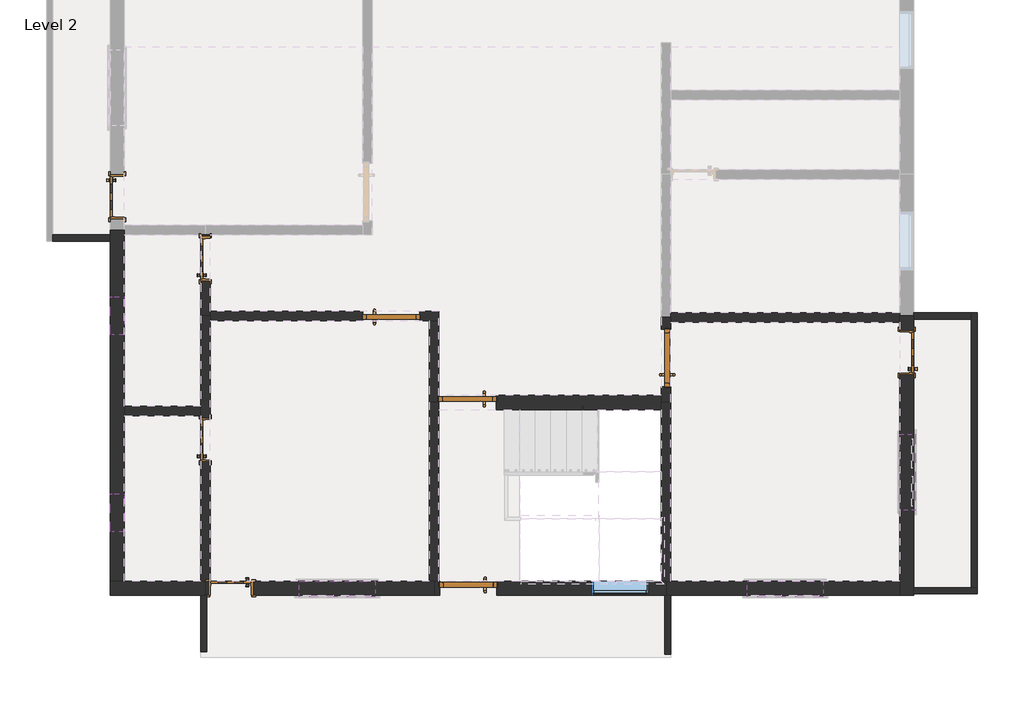
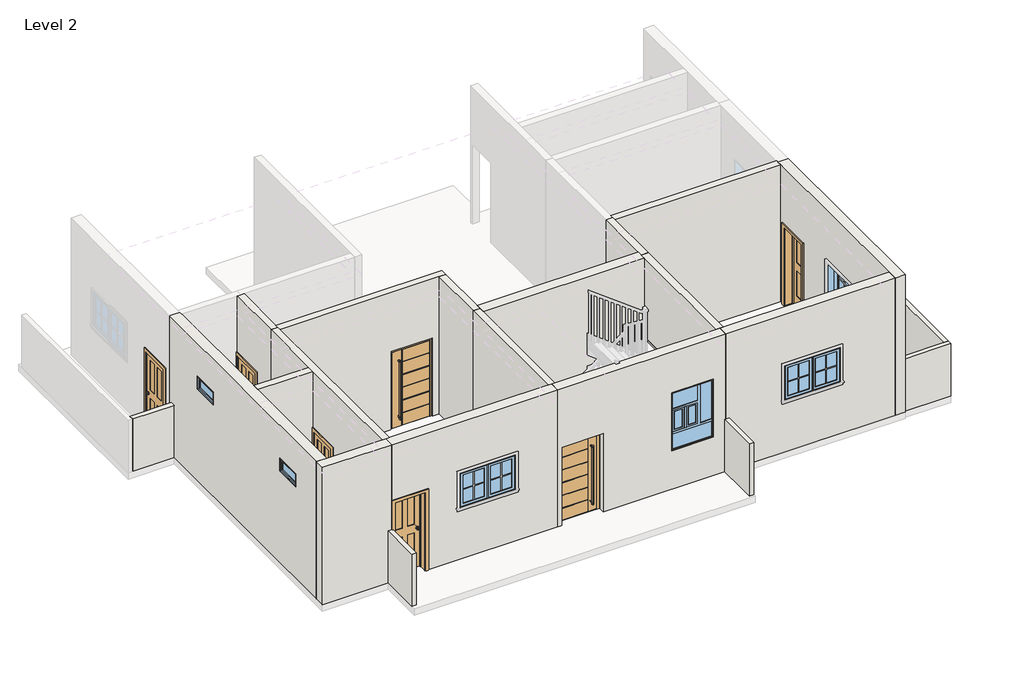
# One storey, part 1 of 3: 22 walls, 9 doors, 6 windows.
"""IFC4 building model written with IfcOpenShell, lengths in millimetres."""

from ifc_helpers import new_model, si_unit, frame, origin, place, context, project, spatial, polyline, outline, extrude, faceted_brep, transform, mapped, element, save
from components import door_3_44036f4b, door_3_3562bf2b, door_a03dd1d4, door_a34dad57, m_fixed_2_dd9f9b20, m_window_awning_double_horizontal_4_8afcb0b2, m_window_casement_double_sash_variable_3_661e274a

model = new_model("IFC4")

# Units and contexts
model_context = context("Model", 3, world=origin())
ifc_project = project(units=[si_unit("LENGTHUNIT", "METRE", prefix="MILLI")], contexts=[model_context])

# Site, building, storey
site = spatial("IfcSite", under=ifc_project)
building = spatial("IfcBuilding", under=site)
storey = spatial("IfcBuildingStorey", under=building, Name="Level 2", Elevation=3200.4)

# Doors
placement = place(None, origin())
door_3_shape = door_3_44036f4b(model_context)
element("IfcDoor", 1, ObjectType="3'", at=placement, inside=storey, context=model_context, shape_type="MappedRepresentation", body=[
    mapped(door_3_shape, transform((-13795.5794909, -9.3618509, 3200.4), x_axis=(1.0, 0.0, 0.0), y_axis=(0.0, 1.0, 0.0), z_axis=(0.0, 0.0, 1.0))),
])
element("IfcDoor", 2, ObjectType="3'", at=placement, inside=storey, context=model_context, shape_type="MappedRepresentation", body=[
    mapped(door_3_shape, transform((-9401.3794909, -682.4618509, 3200.4), x_axis=(0.0, 1.0, 0.0), y_axis=(-1.0, 0.0, 0.0), z_axis=(0.0, 0.0, 1.0))),
])
door_3_2_shape = door_3_3562bf2b(model_context)
element("IfcDoor", 3, ObjectType="3'", at=placement, inside=storey, context=model_context, shape_type="MappedRepresentation", body=[
    mapped(door_3_2_shape, transform((-12576.3794909, -1393.6618509, 3200.4), x_axis=(-1.0, 0.0, 0.0), y_axis=(0.0, -1.0, 0.0), z_axis=(0.0, 0.0, 1.0))),
])
element("IfcDoor", 4, ObjectType="3'", at=placement, inside=storey, context=model_context, shape_type="MappedRepresentation", body=[
    mapped(door_3_2_shape, transform((-12563.6794909, -4365.4618509, 3200.4), x_axis=(-1.0, 0.0, 0.0), y_axis=(0.0, -1.0, 0.0), z_axis=(0.0, 0.0, 1.0))),
])
door_shape = door_a03dd1d4(model_context)
element("IfcDoor", 5, ObjectType="M_Door-Interior-Single-4_Panel-Wood : 2'2\"", at=placement, inside=storey, context=model_context, shape_type="MappedRepresentation", body=[
    mapped(door_shape, transform((-16770.5544909, -1990.1618509, 3200.4), x_axis=(0.0, 1.0, 0.0), y_axis=(-1.0, 0.0, 0.0), z_axis=(0.0, 0.0, 1.0))),
])
element("IfcDoor", 6, ObjectType="M_Door-Interior-Single-4_Panel-Wood : 2'2\"", at=placement, inside=storey, context=model_context, shape_type="MappedRepresentation", body=[
    mapped(door_shape, transform((-16770.5544909, 905.4381491, 3200.4), x_axis=(0.0, 1.0, 0.0), y_axis=(-1.0, 0.0, 0.0), z_axis=(0.0, 0.0, 1.0))),
])
door_2_shape = door_a34dad57(model_context)
element("IfcDoor", 7, ObjectType="M_Door-Interior-Single-4_Panel-Wood : 2'2\"", at=placement, inside=storey, context=model_context, shape_type="MappedRepresentation", body=[
    mapped(door_2_shape, transform((-18180.2544909, 1895.2381491, 3200.4), x_axis=(0.0, -1.0, 0.0), y_axis=(1.0, 0.0, 0.0), z_axis=(0.0, 0.0, 1.0))),
])
element("IfcDoor", 8, ObjectType="M_Door-Interior-Single-4_Panel-Wood : 2'2\"", at=placement, inside=storey, context=model_context, shape_type="MappedRepresentation", body=[
    mapped(door_2_shape, transform((-5550.1044909, -593.1618509, 3200.4), x_axis=(0.0, 1.0, 0.0), y_axis=(-1.0, 0.0, 0.0), z_axis=(0.0, 0.0, 1.0))),
])
element("IfcDoor", 9, ObjectType="M_Door-Interior-Single-4_Panel-Wood : 2'2\"", at=placement, inside=storey, context=model_context, shape_type="MappedRepresentation", body=[
    mapped(door_2_shape, transform((-16361.3794909, -4362.2868509, 3200.4), x_axis=(-1.0, 0.0, 0.0), y_axis=(0.0, -1.0, 0.0), z_axis=(0.0, 0.0, 1.0))),
])

# Walls
element("IfcWall", 10, ObjectType="Generic - 4\"", at=placement, inside=storey, context=model_context, shape_type="Brep", body=[
    faceted_brep([(-16843.5794909, -4479.7618509, 3200.4), (-16843.5794909, -5381.4618509, 3200.4), (-16843.5794909, -5381.4618509, 4419.6), (-16843.5794909, -4479.7618509, 4419.6), (-16741.9794909, -4479.7618509, 3200.4), (-16741.9794909, -4479.7618509, 4419.6), (-16741.9794909, -5381.4618509, 4419.6), (-16741.9794909, -5381.4618509, 3200.4), (-16767.3794909, -4479.7618509, 3200.4)], [[[0, 1, 2, 3]], [[4, 5, 6, 7]], [[1, 0, 8, 4, 7]], [[2, 1, 7, 6]], [[3, 2, 6, 5]], [[0, 3, 5, 4, 8]]]),
])
element("IfcWall", 11, ObjectType="Generic - 4\"", at=placement, inside=storey, context=model_context, shape_type="Brep", body=[
    faceted_brep([(-9325.1794909, -5419.5618509, 3200.4), (-9325.1794909, -4479.7618509, 3200.4), (-9325.1794909, -4479.7618509, 4419.6), (-9325.1794909, -5419.5618509, 4419.6), (-9426.7794909, -5419.5618509, 3200.4), (-9426.7794909, -5419.5618509, 4419.6), (-9426.7794909, -4479.7618509, 4419.6), (-9426.7794909, -4479.7618509, 3200.4), (-9401.3794909, -4479.7618509, 3200.4)], [[[0, 1, 2, 3]], [[4, 5, 6, 7]], [[1, 0, 4, 7, 8]], [[3, 2, 6, 5]], [[0, 3, 5, 4]], [[2, 1, 8, 7, 6]]]),
])
element("IfcWall", 12, ObjectType="Generic - 4\"", at=placement, inside=storey, context=model_context, shape_type="Brep", body=[
    faceted_brep([(-5438.9794909, -4454.3618509, 3200.4), (-4422.9794909, -4454.3618509, 3200.4), (-4422.9794909, -4454.3618509, 4419.6), (-5438.9794909, -4454.3618509, 4419.6), (-5438.9794909, -4352.7618509, 3200.4), (-5438.9794909, -4352.7618509, 4419.6), (-4524.5794909, -4352.7618509, 4419.6), (-4422.9794909, -4352.7618509, 4419.6), (-4422.9794909, -4352.7618509, 3200.4), (-4524.5794909, -4352.7618509, 3200.4)], [[[0, 1, 2, 3]], [[4, 5, 6, 7, 8, 9]], [[1, 0, 4, 9, 8]], [[3, 2, 7, 6, 5]], [[0, 3, 5, 4]], [[2, 1, 8, 7]]]),
])
element("IfcWall", 13, ObjectType="Generic - 4\"", at=placement, inside=storey, context=model_context, shape_type="Brep", body=[
    faceted_brep([(-4422.9794909, -4352.7618509, 3200.4), (-4422.9794909, 41.4381491, 3200.4), (-4422.9794909, 41.4381491, 4419.6), (-4422.9794909, -4352.7618509, 4419.6), (-4524.5794909, -4352.7618509, 3200.4), (-4524.5794909, -4352.7618509, 4419.6), (-4524.5794909, -60.1618509, 4419.6), (-4524.5794909, 41.4381491, 4419.6), (-4524.5794909, 41.4381491, 3200.4), (-4524.5794909, -60.1618509, 3200.4)], [[[0, 1, 2, 3]], [[4, 5, 6, 7, 8, 9]], [[1, 0, 4, 9, 8]], [[3, 2, 7, 6, 5]], [[0, 3, 5, 4]], [[2, 1, 8, 7]]]),
])
element("IfcWall", 14, ObjectType="Generic - 4\"", at=placement, inside=storey, context=model_context, shape_type="Brep", body=[
    faceted_brep([(-4524.5794909, 41.4381491, 3200.4), (-5438.9794909, 41.4381491, 3200.4), (-5438.9794909, 41.4381491, 4419.6), (-4524.5794909, 41.4381491, 4419.6), (-4524.5794909, -60.1618509, 3200.4), (-4524.5794909, -60.1618509, 4419.6), (-5438.9794909, -60.1618509, 4419.6), (-5438.9794909, -60.1618509, 3200.4), (-5438.9794909, -9.3618509, 3200.4)], [[[0, 1, 2, 3]], [[4, 5, 6, 7]], [[1, 0, 4, 7, 8]], [[3, 2, 6, 5]], [[0, 3, 5, 4]], [[2, 1, 8, 7, 6]]]),
])
element("IfcWall", 15, ObjectType="Generic - 4\"", at=placement, inside=storey, context=model_context, shape_type="SweptSolid", body=[
    extrude(outline(polyline([(-18291.3794909, 1184.4381491), (-19205.7794909, 1184.4381491), (-19205.7794909, 1286.0381491), (-18291.3794909, 1286.0381491), (-18291.3794909, 1184.4381491)])), frame((0.0, 0.0, 3200.4), z_axis=(0.0, 0.0, 1.0), x_axis=(1.0, 0.0, 0.0)), (0.0, 0.0, 1.0), 1219.2),
])
element("IfcWall", 16, ObjectType="Generic - 6\"", at=placement, inside=storey, context=model_context, shape_type="Brep", body=[
    faceted_brep([(-16691.1794909, -9.3618509, 3200.4), (-16691.1794909, -9.3618509, 6400.8), (-16691.1794909, -85.5618509, 6400.8), (-16691.1794909, -4251.1618509, 6400.8), (-16691.1794909, -4251.1618509, 3200.4), (-16691.1794909, -2345.3618509, 3200.4), (-16691.1794909, -2345.3618509, 5054.2), (-16691.1794909, -1634.9618509, 5054.2), (-16691.1794909, -1634.9618509, 3200.4), (-16691.1794909, -85.5618509, 3200.4), (-16843.5794909, -9.3618509, 6400.8), (-16843.5794909, -9.3618509, 3200.4), (-16843.5794909, -1457.1618509, 3200.4), (-16843.5794909, -1609.5618509, 3200.4), (-16843.5794909, -1634.9618509, 3200.4), (-16843.5794909, -1634.9618509, 5054.2), (-16843.5794909, -2345.3618509, 5054.2), (-16843.5794909, -2345.3618509, 3200.4), (-16843.5794909, -4251.1618509, 3200.4), (-16843.5794909, -4251.1618509, 6400.8), (-16843.5794909, -1609.5618509, 6400.8), (-16843.5794909, -1457.1618509, 6400.8), (-16716.5794909, -4251.1618509, 3200.4), (-16767.3794909, -4251.1618509, 3200.4), (-16767.3794909, -4251.1618509, 6400.8)], [[[0, 1, 2, 3, 4, 5, 6, 7, 8, 9]], [[10, 11, 12, 13, 14, 15, 16, 17, 18, 19, 20, 21]], [[4, 22, 23, 18, 17, 5]], [[11, 0, 9, 8, 14, 13, 12]], [[1, 0, 11, 10]], [[3, 2, 1, 10, 21, 20, 19, 24]], [[7, 15, 14, 8]], [[15, 7, 6, 16]], [[16, 6, 5, 17]], [[3, 24, 19, 18, 23, 22, 4]]]),
])
element("IfcWall", 17, ObjectType="Generic - 6\"", at=placement, inside=storey, context=model_context, shape_type="SweptSolid", body=[
    extrude(outline(polyline([(-16843.5794909, -1609.5618509), (-18062.7794909, -1609.5618509), (-18062.7794909, -1457.1618509), (-16843.5794909, -1457.1618509), (-16843.5794909, -1609.5618509)])), frame((0.0, 0.0, 3200.4), z_axis=(0.0, 0.0, 1.0), x_axis=(1.0, 0.0, 0.0)), (0.0, 0.0, 1.0), 3200.4),
])
element("IfcWall", 18, ObjectType="Generic - 6\"", at=placement, inside=storey, context=model_context, shape_type="Brep", body=[
    faceted_brep([(-13033.5794909, -85.5618509, 6400.8), (-13185.9794909, -85.5618509, 6400.8), (-16691.1794909, -85.5618509, 6400.8), (-16691.1794909, -85.5618509, 3200.4), (-14252.7794909, -85.5618509, 3200.4), (-14252.7794909, -85.5618509, 5029.2), (-13338.3794909, -85.5618509, 5029.2), (-13338.3794909, -85.5618509, 3200.4), (-13185.9794909, -85.5618509, 3200.4), (-13033.5794909, -85.5618509, 3200.4), (-16691.1794909, 66.8381491, 6400.8), (-13033.5794909, 66.8381491, 6400.8), (-13033.5794909, 66.8381491, 3200.4), (-13338.3794909, 66.8381491, 3200.4), (-13338.3794909, 66.8381491, 5029.2), (-14252.7794909, 66.8381491, 5029.2), (-14252.7794909, 66.8381491, 3200.4), (-16691.1794909, 66.8381491, 3200.4), (-13338.3794909, -65.5618509, 3200.4), (-13323.3794909, -65.5618509, 3200.4), (-13323.3794909, 11.4381491, 3200.4), (-13338.3794909, 11.4381491, 3200.4), (-16691.1794909, -9.3618509, 3200.4), (-14252.7794909, 11.4381491, 3200.4), (-14267.7794909, 11.4381491, 3200.4), (-14267.7794909, -65.5618509, 3200.4), (-14252.7794909, -65.5618509, 3200.4), (-16691.1794909, -9.3618509, 6400.8), (-14252.7794909, -65.5618509, 5029.2), (-13338.3794909, -65.5618509, 5029.2), (-13338.3794909, 11.4381491, 5029.2), (-14252.7794909, 11.4381491, 5029.2), (-14267.7794909, -65.5618509, 5044.2), (-14267.7794909, 11.4381491, 5044.2), (-13323.3794909, 11.4381491, 5044.2), (-13323.3794909, -65.5618509, 5044.2)], [[[0, 1, 2, 3, 4, 5, 6, 7, 8, 9]], [[10, 11, 12, 13, 14, 15, 16, 17]], [[12, 9, 8, 7, 18, 19, 20, 21, 13]], [[3, 22, 17, 16, 23, 24, 25, 26, 4]], [[2, 1, 0, 11, 10, 27]], [[3, 2, 27, 10, 17, 22]], [[0, 9, 12, 11]], [[5, 28, 29, 6]], [[14, 30, 31, 15]], [[6, 29, 18, 7]], [[30, 14, 13, 21]], [[28, 5, 4, 26]], [[15, 31, 23, 16]], [[32, 33, 34, 35]], [[35, 34, 20, 19]], [[31, 30, 21, 20, 34, 33, 24, 23]], [[33, 32, 25, 24]], [[29, 28, 26, 25, 32, 35, 19, 18]]]),
])
element("IfcWall", 19, ObjectType="Generic - 6\"", at=placement, inside=storey, context=model_context, shape_type="Brep", body=[
    faceted_brep([(-13185.9794909, -85.5618509, 3200.4), (-13185.9794909, -1393.6618509, 3200.4), (-13185.9794909, -1393.6618509, 6400.8), (-13185.9794909, -85.5618509, 6400.8), (-13033.5794909, -85.5618509, 6400.8), (-13033.5794909, -1279.3618509, 6400.8), (-13033.5794909, -1393.6618509, 6400.8), (-13033.5794909, -1393.6618509, 5029.2), (-13033.5794909, -1393.6618509, 3200.4), (-13033.5794909, -1376.3618508, 3200.4), (-13033.5794909, -1376.3618508, 5029.2), (-13033.5794909, -1376.3618508, 5044.2), (-13033.5794909, -1299.3618508, 5044.2), (-13033.5794909, -1299.3618508, 5029.2), (-13033.5794909, -1299.3618508, 3200.4), (-13033.5794909, -1279.3618508, 3200.4), (-13033.5794909, -85.5618509, 3200.4), (-13048.5794909, -1299.3618508, 3200.4), (-13048.5794909, -1376.3618508, 3200.4), (-13048.5794909, -1376.3618508, 5044.2), (-13048.5794909, -1299.3618508, 5044.2)], [[[0, 1, 2, 3]], [[4, 5, 6, 7, 8, 9, 10, 11, 12, 13, 14, 15, 16]], [[1, 0, 16, 15, 14, 17, 18, 9, 8]], [[2, 1, 8, 7, 6]], [[3, 2, 6, 5, 4]], [[0, 3, 4, 16]], [[19, 20, 12, 11]], [[20, 19, 18, 17]], [[18, 19, 11, 10, 9]], [[20, 17, 14, 13, 12]]]),
])
element("IfcWall", 20, ObjectType="Generic - 6\"", at=placement, inside=storey, context=model_context, shape_type="Brep", body=[
    faceted_brep([(-9325.1794909, -4251.1618509, 6400.8), (-9325.1794909, -4251.1618509, 3200.4), (-9325.1794909, -1393.6618509, 3200.4), (-9325.1794909, -1393.6618509, 6400.8), (-9477.5794909, -4251.1618509, 3200.4), (-9477.5794909, -4251.1618509, 6400.8), (-9477.5794909, -1507.9618509, 6400.8), (-9477.5794909, -1393.6618509, 6400.8), (-9477.5794909, -1393.6618509, 3200.4), (-9477.5794909, -1507.9618509, 3200.4), (-9401.3794909, -4251.1618509, 3200.4), (-9401.3794909, -4251.1618509, 6400.8)], [[[0, 1, 2, 3]], [[4, 5, 6, 7, 8, 9]], [[2, 1, 10, 4, 9, 8]], [[3, 2, 8, 7]], [[0, 3, 7, 6, 5, 11]], [[0, 11, 5, 4, 10, 1]]]),
])
element("IfcWall", 21, ObjectType="Generic - 6\"", at=placement, inside=storey, context=model_context, shape_type="Brep", body=[
    faceted_brep([(-5667.5794909, 41.4381491, 3200.4), (-9325.1794909, 41.4381491, 3200.4), (-9325.1794909, 41.4381491, 6400.8), (-5667.5794909, 41.4381491, 6400.8), (-5667.5794909, -110.9618509, 3200.4), (-5667.5794909, -110.9618509, 6400.8), (-9325.1794909, -110.9618509, 6400.8), (-9325.1794909, -110.9618509, 3200.4), (-5667.5794909, -9.3618509, 3200.4), (-9325.1794909, -34.7618509, 3200.4), (-9325.1794909, -34.7618509, 6400.8), (-5667.5794909, -9.3618509, 6400.8)], [[[0, 1, 2, 3]], [[4, 5, 6, 7]], [[1, 0, 8, 4, 7, 9]], [[3, 2, 10, 6, 5, 11]], [[0, 3, 11, 5, 4, 8]], [[2, 1, 9, 7, 6, 10]]]),
])
element("IfcWall", 22, ObjectType="Generic - 6\"", at=placement, inside=storey, context=model_context, shape_type="Brep", body=[
    faceted_brep([(-16691.1794909, 1286.0381491, 6400.8), (-16691.1794909, 66.8381491, 6400.8), (-16691.1794909, -9.3618509, 6400.8), (-16691.1794909, -9.3618509, 3200.4), (-16691.1794909, 66.8381491, 3200.4), (-16691.1794909, 550.2381491, 3200.4), (-16691.1794909, 550.2381491, 5054.2), (-16691.1794909, 1260.6381491, 5054.2), (-16691.1794909, 1260.6381491, 3200.4), (-16691.1794909, 1286.0381491, 3200.4), (-16843.5794909, -9.3618509, 6400.8), (-16843.5794909, 1286.0381491, 6400.8), (-16843.5794909, 1286.0381491, 3200.4), (-16843.5794909, 1260.6381491, 3200.4), (-16843.5794909, 1260.6381491, 5054.2), (-16843.5794909, 550.2381491, 5054.2), (-16843.5794909, 550.2381491, 3200.4), (-16843.5794909, -9.3618509, 3200.4), (-16767.3794909, 1286.0381491, 3200.4), (-16767.3794909, 1286.0381491, 6400.8)], [[[0, 1, 2, 3, 4, 5, 6, 7, 8, 9]], [[10, 11, 12, 13, 14, 15, 16, 17]], [[12, 18, 9, 8, 13]], [[3, 17, 16, 5, 4]], [[2, 1, 0, 19, 11, 10]], [[3, 2, 10, 17]], [[0, 9, 18, 12, 11, 19]], [[7, 14, 13, 8]], [[14, 7, 6, 15]], [[15, 6, 5, 16]]]),
])
element("IfcWall", 23, ObjectType="Generic - 6\"", at=placement, inside=storey, context=model_context, shape_type="Brep", body=[
    faceted_brep([(-9325.1794909, -34.7618509, 3200.4), (-9325.1794909, -34.7618509, 6400.8), (-9325.1794909, -110.9618509, 6400.8), (-9325.1794909, -1393.6618509, 6400.8), (-9325.1794909, -1393.6618509, 3200.4), (-9325.1794909, -1139.6618509, 3200.4), (-9325.1794909, -1139.6618509, 5029.2), (-9325.1794909, -225.2618509, 5029.2), (-9325.1794909, -225.2618509, 3200.4), (-9325.1794909, -110.9618509, 3200.4), (-9477.5794909, -34.7618509, 6400.8), (-9477.5794909, -34.7618509, 3200.4), (-9477.5794909, -225.2618509, 3200.4), (-9477.5794909, -225.2618509, 5029.2), (-9477.5794909, -1139.6618509, 5029.2), (-9477.5794909, -1139.6618509, 3200.4), (-9477.5794909, -1279.3618509, 3200.4), (-9477.5794909, -1393.6618509, 3200.4), (-9477.5794909, -1393.6618509, 6400.8), (-9477.5794909, -1279.3618509, 6400.8), (-9345.1794909, -225.2618509, 3200.4), (-9345.1794909, -210.2618509, 3200.4), (-9422.1794909, -210.2618509, 3200.4), (-9422.1794909, -225.2618509, 3200.4), (-9422.1794909, -1139.6618509, 3200.4), (-9422.1794909, -1154.6618509, 3200.4), (-9345.1794909, -1154.6618509, 3200.4), (-9345.1794909, -1139.6618509, 3200.4), (-9345.1794909, -1139.6618509, 5029.2), (-9345.1794909, -225.2618509, 5029.2), (-9422.1794909, -225.2618509, 5029.2), (-9422.1794909, -1139.6618509, 5029.2), (-9345.1794909, -1154.6618509, 5044.2), (-9422.1794909, -1154.6618509, 5044.2), (-9422.1794909, -210.2618509, 5044.2), (-9345.1794909, -210.2618509, 5044.2)], [[[0, 1, 2, 3, 4, 5, 6, 7, 8, 9]], [[10, 11, 12, 13, 14, 15, 16, 17, 18, 19]], [[11, 0, 9, 8, 20, 21, 22, 23, 12]], [[4, 17, 16, 15, 24, 25, 26, 27, 5]], [[1, 0, 11, 10]], [[3, 2, 1, 10, 19, 18]], [[4, 3, 18, 17]], [[6, 28, 29, 7]], [[13, 30, 31, 14]], [[30, 13, 12, 23]], [[7, 29, 20, 8]], [[14, 31, 24, 15]], [[28, 6, 5, 27]], [[32, 33, 34, 35]], [[35, 34, 22, 21]], [[31, 30, 23, 22, 34, 33, 25, 24]], [[33, 32, 26, 25]], [[29, 28, 27, 26, 32, 35, 21, 20]]]),
])
element("IfcWall", 24, ObjectType="Generic - 6\"", at=placement, inside=storey, context=model_context, shape_type="Brep", body=[
    faceted_brep([(-13185.9794909, -1393.6618509, 3200.4), (-13185.9794909, -4251.1618509, 3200.4), (-13185.9794909, -4251.1618509, 6400.8), (-13185.9794909, -1393.6618509, 6400.8), (-13033.5794909, -1393.6618509, 6400.8), (-13033.5794909, -1507.9618509, 6400.8), (-13033.5794909, -4251.1618509, 6400.8), (-13033.5794909, -4251.1618509, 3200.4), (-13033.5794909, -1507.9618509, 3200.4), (-13033.5794909, -1393.6618509, 3200.4), (-13033.5794909, -1393.6618509, 5029.2), (-13109.7794909, -4251.1618509, 3200.4), (-13109.7794909, -4251.1618509, 6400.8)], [[[0, 1, 2, 3]], [[4, 5, 6, 7, 8, 9, 10]], [[1, 0, 9, 8, 7, 11]], [[3, 2, 12, 6, 5, 4]], [[0, 3, 4, 10, 9]], [[2, 1, 11, 7, 6, 12]]]),
])
element("IfcWall", 25, ObjectType="Generic - 9\"", at=placement, inside=storey, context=model_context, shape_type="Brep", body=[
    faceted_brep([(-5667.5794909, -4251.1618509, 6400.8), (-5667.5794909, -4251.1618509, 3200.4), (-9325.1794909, -4251.1618509, 3200.4), (-9401.3794909, -4251.1618509, 3200.4), (-9401.3794909, -4251.1618509, 6400.8), (-9325.1794909, -4251.1618509, 6400.8), (-8105.9794909, -4251.1618509, 5219.6), (-8105.9794909, -4251.1618509, 4419.6), (-6886.7794909, -4251.1618509, 4419.6), (-6886.7794909, -4251.1618509, 5219.6), (-5667.5794909, -4479.7618509, 3200.4), (-5667.5794909, -4479.7618509, 6400.8), (-9401.3794909, -4479.7618509, 6400.8), (-9401.3794909, -4479.7618509, 3200.4), (-9325.1794909, -4479.7618509, 3200.4), (-8105.9794909, -4479.7618509, 5219.6), (-6886.7794909, -4479.7618509, 5219.6), (-6886.7794909, -4479.7618509, 4419.6), (-8105.9794909, -4479.7618509, 4419.6)], [[[0, 1, 2, 3, 4, 5], [6, 7, 8, 9]], [[10, 11, 12, 13, 14], [15, 16, 17, 18]], [[3, 2, 1, 10, 14, 13]], [[0, 5, 4, 12, 11]], [[0, 11, 10, 1]], [[7, 6, 15, 18]], [[8, 7, 18, 17]], [[9, 8, 17, 16]], [[6, 9, 16, 15]], [[3, 13, 12, 4]]]),
])
element("IfcWall", 26, ObjectType="Generic - 9\"", at=placement, inside=storey, context=model_context, shape_type="Brep", body=[
    faceted_brep([(-18062.7794909, -4251.1618509, 3200.4), (-18062.7794909, -1609.5618509, 3200.4), (-18062.7794909, -1457.1618509, 3200.4), (-18062.7794909, 1286.0381491, 3200.4), (-18062.7794909, 1362.2381491, 3200.4), (-18062.7794909, 1362.2381491, 6400.8), (-18062.7794909, 1286.0381491, 6400.8), (-18062.7794909, -1457.1618509, 6400.8), (-18062.7794909, -1609.5618509, 6400.8), (-18062.7794909, -4251.1618509, 6400.8), (-18062.7794909, -3463.7618509, 5334.0), (-18062.7794909, -3463.7618509, 5638.8), (-18062.7794909, -2854.1618509, 5638.8), (-18062.7794909, -2854.1618509, 5334.0), (-18062.7794909, -314.1618509, 5334.0), (-18062.7794909, -314.1618509, 5638.8), (-18062.7794909, 295.4381491, 5638.8), (-18062.7794909, 295.4381491, 5334.0), (-18291.3794909, -4251.1618509, 3200.4), (-18291.3794909, -4251.1618509, 6400.8), (-18291.3794909, 1362.2381491, 6400.8), (-18291.3794909, 1362.2381491, 3200.4), (-18291.3794909, 1286.0381491, 3200.4), (-18291.3794909, 1184.4381491, 3200.4), (-18291.3794909, -3463.7618509, 5334.0), (-18291.3794909, -2854.1618509, 5334.0), (-18291.3794909, -2854.1618509, 5638.8), (-18291.3794909, -3463.7618509, 5638.8), (-18291.3794909, -314.1618509, 5334.0), (-18291.3794909, 295.4381491, 5334.0), (-18291.3794909, 295.4381491, 5638.8), (-18291.3794909, -314.1618509, 5638.8)], [[[0, 1, 2, 3, 4, 5, 6, 7, 8, 9], [10, 11, 12, 13], [14, 15, 16, 17]], [[18, 19, 20, 21, 22, 23], [24, 25, 26, 27], [28, 29, 30, 31]], [[4, 3, 2, 1, 0, 18, 23, 22, 21]], [[5, 4, 21, 20]], [[9, 8, 7, 6, 5, 20, 19]], [[0, 9, 19, 18]], [[11, 10, 24, 27]], [[12, 11, 27, 26]], [[13, 12, 26, 25]], [[10, 13, 25, 24]], [[15, 14, 28, 31]], [[16, 15, 31, 30]], [[17, 16, 30, 29]], [[14, 17, 29, 28]]]),
])
element("IfcWall", 27, ObjectType="Generic - 9\"", at=placement, inside=storey, context=model_context, shape_type="Brep", body=[
    faceted_brep([(-13033.5794909, -1279.3618509, 6400.8), (-9477.5794909, -1279.3618509, 6400.8), (-9477.5794909, -1279.3618509, 3200.4), (-12119.1794909, -1279.3618509, 3200.4), (-12119.1794909, -1279.3618509, 5029.2), (-13033.5794909, -1279.3618509, 5029.2), (-9477.5794909, -1507.9618509, 6400.8), (-13033.5794909, -1507.9618509, 6400.8), (-13033.5794909, -1507.9618509, 5029.2), (-12119.1794909, -1507.9618509, 5029.2), (-12119.1794909, -1507.9618509, 3200.4), (-9477.5794909, -1507.9618509, 3200.4), (-9477.5794909, -1393.6618509, 3200.4), (-12119.1794909, -1376.3618508, 3200.4), (-12104.1794909, -1376.3618508, 3200.4), (-12104.1794909, -1299.3618508, 3200.4), (-12119.1794909, -1299.3618508, 3200.4), (-13033.5794909, -1393.6618509, 6400.8), (-9477.5794909, -1393.6618509, 6400.8), (-13033.5794909, -1299.3618508, 5029.2), (-13033.5794909, -1299.3618508, 5044.2), (-13033.5794909, -1376.3618508, 5044.2), (-13033.5794909, -1376.3618508, 5029.2), (-12119.1794909, -1299.3618508, 5029.2), (-12119.1794909, -1376.3618508, 5029.2), (-12104.1794909, -1299.3618508, 5044.2), (-12104.1794909, -1376.3618508, 5044.2)], [[[0, 1, 2, 3, 4, 5]], [[6, 7, 8, 9, 10, 11]], [[2, 12, 11, 10, 13, 14, 15, 16, 3]], [[1, 0, 17, 7, 6, 18]], [[7, 17, 0, 5, 19, 20, 21, 22, 8]], [[2, 1, 18, 6, 11, 12]], [[4, 23, 19, 5]], [[22, 24, 9, 8]], [[23, 4, 3, 16]], [[9, 24, 13, 10]], [[25, 26, 21, 20]], [[24, 22, 21, 26, 14, 13]], [[26, 25, 15, 14]], [[19, 23, 16, 15, 25, 20]]]),
])
element("IfcWall", 28, ObjectType="Generic - 9\"", at=placement, inside=storey, context=model_context, shape_type="Brep", body=[
    faceted_brep([(-5667.5794909, -4479.7618509, 6400.8), (-5667.5794909, -4251.1618509, 6400.8), (-5667.5794909, -110.9618509, 6400.8), (-5667.5794909, -9.3618509, 6400.8), (-5667.5794909, -9.3618509, 3200.4), (-5667.5794909, -110.9618509, 3200.4), (-5667.5794909, -237.9618509, 3200.4), (-5667.5794909, -237.9618509, 5054.2), (-5667.5794909, -948.3618509, 5054.2), (-5667.5794909, -948.3618509, 3200.4), (-5667.5794909, -4251.1618509, 3200.4), (-5667.5794909, -4479.7618509, 3200.4), (-5667.5794909, -3120.0618509, 5219.6), (-5667.5794909, -3120.0618509, 4419.6), (-5667.5794909, -1900.8618509, 4419.6), (-5667.5794909, -1900.8618509, 5219.6), (-5438.9794909, -9.3618509, 6400.8), (-5438.9794909, -4479.7618509, 6400.8), (-5438.9794909, -4479.7618509, 3200.4), (-5438.9794909, -4454.3618509, 3200.4), (-5438.9794909, -4352.7618509, 3200.4), (-5438.9794909, -948.3618509, 3200.4), (-5438.9794909, -948.3618509, 5054.2), (-5438.9794909, -237.9618509, 5054.2), (-5438.9794909, -237.9618509, 3200.4), (-5438.9794909, -60.1618509, 3200.4), (-5438.9794909, -9.3618509, 3200.4), (-5438.9794909, -3120.0618509, 5219.6), (-5438.9794909, -1900.8618509, 5219.6), (-5438.9794909, -1900.8618509, 4419.6), (-5438.9794909, -3120.0618509, 4419.6)], [[[0, 1, 2, 3, 4, 5, 6, 7, 8, 9, 10, 11], [12, 13, 14, 15]], [[16, 17, 18, 19, 20, 21, 22, 23, 24, 25, 26], [27, 28, 29, 30]], [[18, 11, 10, 9, 21, 20, 19]], [[4, 26, 25, 24, 6, 5]], [[3, 2, 1, 0, 17, 16]], [[11, 18, 17, 0]], [[12, 15, 28, 27]], [[15, 14, 29, 28]], [[14, 13, 30, 29]], [[13, 12, 27, 30]], [[3, 16, 26, 4]], [[23, 7, 6, 24]], [[7, 23, 22, 8]], [[8, 22, 21, 9]]]),
])
element("IfcWall", 29, ObjectType="Generic - 9\"", at=placement, inside=storey, context=model_context, shape_type="Brep", body=[
    faceted_brep([(-13109.7794909, -4251.1618509, 3200.4), (-13109.7794909, -4251.1618509, 6400.8), (-13033.5794909, -4251.1618509, 6400.8), (-9477.5794909, -4251.1618509, 6400.8), (-9401.3794909, -4251.1618509, 6400.8), (-9401.3794909, -4251.1618509, 3200.4), (-9477.5794909, -4251.1618509, 3200.4), (-12106.4794909, -4251.1618509, 3200.4), (-12106.4794909, -4251.1618509, 5029.2), (-13020.8794909, -4251.1618509, 5029.2), (-13020.8794909, -4251.1618509, 3200.4), (-13033.5794909, -4251.1618509, 3200.4), (-10595.1794909, -4251.1618509, 5450.4), (-10595.1794909, -4251.1618509, 4100.4), (-9680.7794909, -4251.1618509, 4100.4), (-9680.7794909, -4251.1618509, 5450.4), (-13109.7794909, -4479.7618509, 6400.8), (-13109.7794909, -4479.7618509, 3200.4), (-13020.8794909, -4479.7618509, 3200.4), (-13020.8794909, -4479.7618509, 5029.2), (-12106.4794909, -4479.7618509, 5029.2), (-12106.4794909, -4479.7618509, 3200.4), (-9426.7794909, -4479.7618509, 3200.4), (-9401.3794909, -4479.7618509, 3200.4), (-9401.3794909, -4479.7618509, 6400.8), (-10595.1794909, -4479.7618509, 5450.4), (-9680.7794909, -4479.7618509, 5450.4), (-9680.7794909, -4479.7618509, 4100.4), (-10595.1794909, -4479.7618509, 4100.4), (-12106.4794909, -4348.1618508, 3200.4), (-12091.4794909, -4348.1618508, 3200.4), (-12091.4794909, -4271.1618508, 3200.4), (-12106.4794909, -4271.1618508, 3200.4), (-13020.8794909, -4271.1618508, 3200.4), (-13035.8794909, -4271.1618508, 3200.4), (-13035.8794909, -4348.1618508, 3200.4), (-13020.8794909, -4348.1618508, 3200.4), (-12106.4794909, -4271.1618508, 5029.2), (-13020.8794909, -4271.1618508, 5029.2), (-13020.8794909, -4348.1618508, 5029.2), (-12106.4794909, -4348.1618508, 5029.2), (-12091.4794909, -4271.1618508, 5044.2), (-12091.4794909, -4348.1618508, 5044.2), (-13035.8794909, -4348.1618508, 5044.2), (-13035.8794909, -4271.1618508, 5044.2)], [[[0, 1, 2, 3, 4, 5, 6, 7, 8, 9, 10, 11], [12, 13, 14, 15]], [[16, 17, 18, 19, 20, 21, 22, 23, 24], [25, 26, 27, 28]], [[5, 23, 22, 21, 29, 30, 31, 32, 7, 6]], [[17, 0, 11, 10, 33, 34, 35, 36, 18]], [[1, 0, 17, 16]], [[4, 3, 2, 1, 16, 24]], [[8, 37, 38, 9]], [[19, 39, 40, 20]], [[39, 19, 18, 36]], [[9, 38, 33, 10]], [[20, 40, 29, 21]], [[37, 8, 7, 32]], [[41, 42, 43, 44]], [[44, 43, 35, 34]], [[40, 39, 36, 35, 43, 42, 30, 29]], [[42, 41, 31, 30]], [[38, 37, 32, 31, 41, 44, 34, 33]], [[12, 15, 26, 25]], [[15, 14, 27, 26]], [[14, 13, 28, 27]], [[13, 12, 25, 28]], [[4, 24, 23, 5]]]),
])
element("IfcWall", 30, ObjectType="Generic - 9\"", at=placement, inside=storey, context=model_context, shape_type="Brep", body=[
    faceted_brep([(-16767.3794909, -4251.1618509, 6400.8), (-16691.1794909, -4251.1618509, 6400.8), (-13185.9794909, -4251.1618509, 6400.8), (-13109.7794909, -4251.1618509, 6400.8), (-13109.7794909, -4251.1618509, 3200.4), (-13185.9794909, -4251.1618509, 3200.4), (-16006.1794909, -4251.1618509, 3200.4), (-16006.1794909, -4251.1618509, 5054.2), (-16716.5794909, -4251.1618509, 5054.2), (-16716.5794909, -4251.1618509, 3200.4), (-16767.3794909, -4251.1618509, 3200.4), (-15269.5794909, -4251.1618509, 5219.6), (-15269.5794909, -4251.1618509, 4419.6), (-14050.3794909, -4251.1618509, 4419.6), (-14050.3794909, -4251.1618509, 5219.6), (-13109.7794909, -4479.7618509, 6400.8), (-16767.3794909, -4479.7618509, 6400.8), (-16767.3794909, -4479.7618509, 3200.4), (-16741.9794909, -4479.7618509, 3200.4), (-16716.5794909, -4479.7618509, 3200.4), (-16716.5794909, -4479.7618509, 5054.2), (-16006.1794909, -4479.7618509, 5054.2), (-16006.1794909, -4479.7618509, 3200.4), (-13109.7794909, -4479.7618509, 3200.4), (-15269.5794909, -4479.7618509, 5219.6), (-14050.3794909, -4479.7618509, 5219.6), (-14050.3794909, -4479.7618509, 4419.6), (-15269.5794909, -4479.7618509, 4419.6)], [[[0, 1, 2, 3, 4, 5, 6, 7, 8, 9, 10], [11, 12, 13, 14]], [[15, 16, 17, 18, 19, 20, 21, 22, 23], [24, 25, 26, 27]], [[4, 23, 22, 6, 5]], [[17, 10, 9, 19, 18]], [[3, 2, 1, 0, 16, 15]], [[4, 3, 15, 23]], [[11, 14, 25, 24]], [[14, 13, 26, 25]], [[13, 12, 27, 26]], [[12, 11, 24, 27]], [[8, 20, 19, 9]], [[20, 8, 7, 21]], [[21, 7, 6, 22]], [[10, 17, 16, 0]]]),
])
element("IfcWall", 31, ObjectType="Generic - 9\"", at=placement, inside=storey, context=model_context, shape_type="Brep", body=[
    faceted_brep([(-16767.3794909, -4251.1618509, 6400.8), (-16767.3794909, -4251.1618509, 3200.4), (-16843.5794909, -4251.1618509, 3200.4), (-18062.7794909, -4251.1618509, 3200.4), (-18291.3794909, -4251.1618509, 3200.4), (-18291.3794909, -4251.1618509, 6400.8), (-18062.7794909, -4251.1618509, 6400.8), (-16843.5794909, -4251.1618509, 6400.8), (-16767.3794909, -4479.7618509, 3200.4), (-16767.3794909, -4479.7618509, 6400.8), (-18291.3794909, -4479.7618509, 6400.8), (-18291.3794909, -4479.7618509, 3200.4), (-16843.5794909, -4479.7618509, 3200.4)], [[[0, 1, 2, 3, 4, 5, 6, 7]], [[8, 9, 10, 11, 12]], [[4, 3, 2, 1, 8, 12, 11]], [[0, 7, 6, 5, 10, 9]], [[5, 4, 11, 10]], [[0, 9, 8, 1]]]),
])

# Windows
m_fixed_2_shape = m_fixed_2_dd9f9b20(model_context)
element("IfcWindow", 32, ObjectType="M_Fixed : 2'", at=placement, inside=storey, context=model_context, shape_type="MappedRepresentation", body=[
    mapped(m_fixed_2_shape, transform((-18164.0794909, -3158.9618509, 4419.0), x_axis=(0.0, 1.0, 0.0), y_axis=(-1.0, 0.0, 0.0), z_axis=(0.0, 0.0, 1.0))),
])
element("IfcWindow", 33, ObjectType="M_Fixed : 2'", at=placement, inside=storey, context=model_context, shape_type="MappedRepresentation", body=[
    mapped(m_fixed_2_shape, transform((-18164.0794909, -9.3618509, 4419.0), x_axis=(0.0, 1.0, 0.0), y_axis=(-1.0, 0.0, 0.0), z_axis=(0.0, 0.0, 1.0))),
])
m_window_awning_double_horizontal_4_shape = m_window_awning_double_horizontal_4_8afcb0b2(model_context)
element("IfcWindow", 34, ObjectType="M_Window-Awning-Double-Horizontal : 4'", at=placement, inside=storey, context=model_context, shape_type="MappedRepresentation", body=[
    mapped(m_window_awning_double_horizontal_4_shape, transform((-14659.9794909, -4365.4618509, 3519.6), x_axis=(-1.0, 0.0, 0.0), y_axis=(0.0, -1.0, 0.0), z_axis=(0.0, 0.0, 1.0))),
])
element("IfcWindow", 35, ObjectType="M_Window-Awning-Double-Horizontal : 4'", at=placement, inside=storey, context=model_context, shape_type="MappedRepresentation", body=[
    mapped(m_window_awning_double_horizontal_4_shape, transform((-5553.2794909, -2510.4618509, 3519.6), x_axis=(0.0, -1.0, 0.0), y_axis=(1.0, 0.0, 0.0), z_axis=(0.0, 0.0, 1.0))),
])
element("IfcWindow", 36, ObjectType="M_Window-Awning-Double-Horizontal : 4'", at=placement, inside=storey, context=model_context, shape_type="MappedRepresentation", body=[
    mapped(m_window_awning_double_horizontal_4_shape, transform((-7496.3794909, -4365.4618509, 3519.6), x_axis=(-1.0, 0.0, 0.0), y_axis=(0.0, -1.0, 0.0), z_axis=(0.0, 0.0, 1.0))),
])
m_window_casement_double_sash_variable_3_shape = m_window_casement_double_sash_variable_3_661e274a(model_context)
element("IfcWindow", 37, ObjectType="M_Window-Casement-Double-Sash-Variable : 3'", at=placement, inside=storey, context=model_context, shape_type="MappedRepresentation", body=[
    mapped(m_window_casement_double_sash_variable_3_shape, transform((-10137.9794909, -4365.4618509, 3200.4), x_axis=(-1.0, 0.0, 0.0), y_axis=(0.0, -1.0, 0.0), z_axis=(0.0, 0.0, 1.0))),
])

save(model, "model.ifc")

# Revit data of these elements
# Type "3'"
#   Type Mark = "41"
#   Water resistance = "up to Class E900, EN 12208:2001"
#   Uniclass2015Version = "v1.21"
#   Uniclass2015Reference = "Ss_25_30_20_30"
#   Uniclass2015Description = "Frame and door leaf system"
#   URL = "www.aluprof.com"
#   Type IFC Predefined Type = "USERDEFINED"
#   Right-hand / Left-hand door [instance default] = ""
#   Resistance to wind load = "up to Class C5/B5, EN 12210:2001"
#   Insert type = "ST"
#   Hardware [instance default] = ""
#   Product page = "https://aluprof.com/en/architects/offer/window-and-door-systems/panel-doors#visualisation"
#   Operation = "SinglePanelOutwardOpening"
#   Opening type = "Outward"
#   NBSReference = "25-50-20/125"
#   NBSDescription = "Frame and door leaf system"
#   Important = "The actual acceptable construction dimensions are dependent on the selection of profiles and hardware, glazing type, construction weight and the construction’s operating conditions. These should be determined by a suitably qualified person, and using ALUPROF’s calculation software"
#   IfcExportType = "USERDEFINED"
#   IfcExportAs = "IfcDoorType"
#   Handle type [instance default] = ""
#   Manufacturer = "ALUPROF SA"
#   Export Type to IFC As = "IfcDoorType"
#   Door sill type [instance default] = ""
#   Description = "External single-leaf panel door outward opening"
#   Model = "MB-86 ST Panel Door AD07"
#   Content of the recyclate in the material = "69.2%"
#   COBie.Type.WarrantyDurationParts = ""
#   COBie.Type.Name = ""
#   COBie.Type.Manufacturer = "ALUPROF SA"
#   COBie.Space.Name = ""
#   COBie.Floor.Name = ""
#   COBie.Facility.Name = ""
#   COBie.CreatedOn = ""
#   COBie.Component.WarrantyStartDate = ""
#   COBie.Component.Name = "MB-86 ST Panel Door AD07"
#   Burglar resistance = "RC2"
#   Air permeability = "up to Class 4, EN 12207:2001"
#   Width of the active leaf = 2' - 8.17717"
#   Placement in wall = 0' - 0.7874"
#   Thickness = 0' - 3.0315"
#   Height of the opening sash = 5' - 9.44094"
#   Handle Offset = 3' - 5.33858"
#   Rough Height = 6' - 2.40945"
#   Rough Width = 3' - 1.1811"
#   Height = 6' - 0"
#   Width = 3' - 0"
#   Construction depth = 0' - 3.0315"
#   Clear opening width = 2' - 3.94882"
#   Clear opening height = 5' - 8.47638"
#   Height of the array = 0' - 11.08136"
#   Schedule No. [instance default] = 1
#   Handrail [instance default] = yes
#   IsExternal = yes
#   Handle [instance default] = no
#   Door closer [instance default] = no
#   Function = 1
#   COBie.Type = yes
#   COBie = yes
#   Access control [instance default] = no
#   Panel = element 361060
#   Wall Closure = (empty or 0)
# Type "M_Door-Interior-Single-4_Panel-Wood : 2'2\""
#   Type Mark = "43"
#   Assembly Code = "C1020300"
#   Analytic Construction = "Wooden"
#   Top Rail = 0' - 4.72441"
#   Thickness = 0' - 1.37795"
#   Thermal Resistance (R) = 0.455703 (m²·K)/W
#   Swing Angle [instance default] = 90.00°
#   Stiles = 0' - 4.72441"
#   Rough Width = 2' - 3.9685"
#   Rough Height = 6' - 0.98425"
#   Mullion = 0' - 4.52756"
#   Lock Rail = 0' - 7.87402"
#   Height = 6' - 0"
#   Width = 2' - 2"
#   Heat Transfer Coefficient (U) = 2.19465 W/(m²·K)
#   Bottom Rail = 0' - 9.05512"
#   Trim Material = Cherry
#   Panel Material = Cherry
#   Frame Material = Cherry
#   Door Handle Material = Aluminum
#   Visual Light Transmittance = 0
#   Solar Heat Gain Coefficient = 0
#   Wall Closure = (empty or 0)
#   Function = (empty or 0)
# Type "Generic - 4\""
#   Layers, outside or top first: 0' - 4" no material (function 1)
# Type "Generic - 6\""
#   Layers, outside or top first: 0' - 6" no material (function 1)
# Type "Generic - 9\""
#   Layers, outside or top first: 0' - 9" no material (function 1)
# Type "M_Fixed : 2'"
#   Type Mark = "37"
#   Construction Type Id = "GSP4R"
#   Analytic Construction = "1/8 in Pilkington single glazing"
#   Visual Light Transmittance = 0.9
#   Thermal Resistance (R) = 0.271106 (m²·K)/W
#   Solar Heat Gain Coefficient = 0.78
#   Heat Transfer Coefficient (U) = 3.6886 W/(m²·K)
#   Height = 1' - 0"
#   Default Sill Height = 3' - 0.02362"
#   Width = 2' - 0"
#   Window Inset = 0' - 0.74803"
#   Define Thermal Properties by = 1
#   Frame Exterior Material = Sash
#   Frame Interior Material = Sash
#   Glass Pane Material = Glass
#   Sash = Sash
#   Wall Closure = (empty or 0)
# Type "M_Window-Awning-Double-Horizontal : 4'"
#   Type Mark = "28"
#   Fire Rating = "0.5h"
#   Assembly Code = "B2020100"
#   Analytic Construction = "Double glazing - domestic"
#   Window Inset [instance default] = 0' - 0"
#   Wall Thickness [instance default] = 0' - 5.90551"
#   Interior Wall Closure [instance default] = 0' - 2.15551"
#   Half Width = 2' - 0"
#   Visual Light Transmittance = 0.81
#   Thermal Resistance (R) = 0.319569 (m²·K)/W
#   Solar Heat Gain Coefficient = 0.76
#   Rough Width = 4' - 0.59055"
#   Rough Height = 2' - 8.08661"
#   Height = 2' - 7.49606"
#   Heat Transfer Coefficient (U) = 3.12929 W/(m²·K)
#   Frame Extension [instance default] = 0' - 0 1/4"
#   Exterior Wall Closure [instance default] = 0' - 1 1/4"
#   Extension Jamb [instance default] = 0' - 2.15551"
#   Default Sill Height = 2' - 11.43307"
#   Width = 4' - 0"
#   Muntin Visibility = yes
#   Interior Trim Visibility [instance default] = yes
#   Exterior Trim Visibility [instance default] = yes
#   Extension Jamb Visibility [instance default] = yes
#   Interior Trim Material = Wood - Stained
#   Muntin Pattern = M_Muntin Pattern_2x2 : M_Muntin Pattern_2x2
#   Interior Trim = M_Trim-Window-Interior-Flat : Picture Frame
#   Interior Frame Material = Wood - Stained
#   Glass Panel Material = Glass
#   Exterior Trim Material = Clad - White
#   Exterior Trim = M_Trim-Window-Exterior-Flat : with Sill
#   Exterior Frame Material = Clad - White
#   Wall Closure = (empty or 0)
# Type "M_Window-Casement-Double-Sash-Variable : 3'"
#   Type Mark = "36"
#   Fire Rating = "0.5h"
#   Assembly Code = "B2020100"
#   Analytic Construction = "Double glazing - domestic"
#   Window Inset [instance default] = 0' - 0 5/8"
#   Wall Thickness [instance default] = 0' - 5.90551"
#   Visual Light Transmittance = 0.81
#   Transom Height Ratio = 0.3
#   Transom Height = 1' - 3.94488"
#   Thermal Resistance (R) = 0.319569 (m²·K)/W
#   Solar Heat Gain Coefficient = 0.76
#   Rough Width = 3' - 0.59055"
#   Rough Height = 4' - 5.74016"
#   Opening Window Height = 1' - 9.25984"
#   Heat Transfer Coefficient (U) = 3.12929 W/(m²·K)
#   Height = 4' - 5.14961"
#   Frame Gap 3 [instance default] = 0' - 1.65041"
#   Frame Gap 2 [instance default] = 0' - 0.62598"
#   Frame Gap 1 = 0' - 1 51/128"
#   Window Width = 1' - 0"
#   Default Sill Height = 2' - 11.43307"
#   Width = 3' - 0"
#   Frame Material = Metal - Aluminum
#   Glass Panel Material = Glass
#   Wall Closure = (empty or 0)
# Elements 1, 2, 3, 4 (IfcDoor, "3'")
#   Right-hand / Left-hand door = ""
#   Hardware = ""
#   Handle type = ""
#   Door sill type = ""
#   Schedule No. = 1
#   Handrail = yes
#   Handle = no
#   Door closer = no
#   Access control = no
#   Phase Created = New Construction
# Elements 5, 6, 7, 8, 9 (IfcDoor, "M_Door-Interior-Single-4_Panel-Wood : 2'2\"")
#   Swing Angle = 90.00°
#   Phase Created = New Construction
#   Materials on its faces: "Cherry", "Aluminum"
# Elements 10, 11, 12, 13, 14, 15 (IfcWall, "Generic - 4\"")
#   Top Offset = 0' - 0"
#   Base Offset = 0' - 0"
#   Unconnected Height = 4' - 0"
#   wall height = 4' - 0"
#   Phase Created = New Construction
#   Base Constraint = Level 2
#   Materials on its faces: "Default Wall", "WALL2"
# Element 16 (IfcWall, "Generic - 6\"")
#   Top Offset = 0' - 0"
#   Base Offset = 0' - 0"
#   Unconnected Height = 10' - 6"
#   wall height = 10' - 6"
#   Phase Created = New Construction
#   Base Constraint = Level 2
#   Materials on its faces: "Default Wall", "BED ROOM WALL 2", "BATH ROOM WALL 1"
# Element 17 (IfcWall, "Generic - 6\"")
#   Top Offset = 0' - 0"
#   Base Offset = 0' - 0"
#   Unconnected Height = 10' - 6"
#   wall height = 10' - 6"
#   Phase Created = New Construction
#   Base Constraint = Level 2
#   Materials on its faces: "Default Wall", "BATH ROOM WALL 1"
# Element 18 (IfcWall, "Generic - 6\"")
#   Top Offset = 0' - 0"
#   Base Offset = 0' - 0"
#   Unconnected Height = 10' - 6"
#   wall height = 10' - 6"
#   Phase Created = New Construction
#   Base Constraint = Level 2
#   Materials on its faces: "Default Wall", "LIVING 2", "BED ROOM WALL1"
# Elements 19, 23 (IfcWall, "Generic - 6\"")
#   Top Offset = 0' - 0"
#   Base Offset = 0' - 0"
#   Unconnected Height = 10' - 6"
#   wall height = 10' - 6"
#   Phase Created = New Construction
#   Base Constraint = Level 2
#   Materials on its faces: "Default Wall", "BED ROOM WALL 2", "LIVING 2"
# Elements 20, 24 (IfcWall, "Generic - 6\"")
#   Top Offset = 0' - 0"
#   Base Offset = 0' - 0"
#   Unconnected Height = 10' - 6"
#   wall height = 10' - 6"
#   Phase Created = New Construction
#   Base Constraint = Level 2
#   Materials on its faces: "Default Wall", "BED ROOM WALL 2", "LIVING"
# Element 21 (IfcWall, "Generic - 6\"")
#   Top Offset = 0' - 0"
#   Base Offset = 0' - 0"
#   Unconnected Height = 10' - 6"
#   wall height = 10' - 6"
#   Phase Created = New Construction
#   Base Constraint = Level 2
#   Materials on its faces: "Default Wall", "LIVING", "BED ROOM WALL1"
# Element 22 (IfcWall, "Generic - 6\"")
#   Top Offset = 0' - 0"
#   Base Offset = 0' - 0"
#   Unconnected Height = 10' - 6"
#   wall height = 10' - 6"
#   Phase Created = New Construction
#   Base Constraint = Level 2
#   Materials on its faces: "Default Wall", "LIVING 2", "BATH ROOM WALL 1"
# Element 25 (IfcWall, "Generic - 9\"")
#   Top Offset = 0' - 0"
#   Base Offset = 0' - 0"
#   Unconnected Height = 10' - 6"
#   wall height = 10' - 6"
#   Phase Created = New Construction
#   Base Constraint = Level 2
#   Materials on its faces: "Default Wall", "BED ROOM WALL 2", "WALL2"
# Element 26 (IfcWall, "Generic - 9\"")
#   Top Offset = 0' - 0"
#   Base Offset = 0' - 0"
#   Unconnected Height = 10' - 6"
#   wall height = 10' - 6"
#   Phase Created = New Construction
#   Base Constraint = Level 2
#   Materials on its faces: "Default Wall", "BATH ROOM WALL 1", "WALL2"
# Element 27 (IfcWall, "Generic - 9\"")
#   Top Offset = 0' - 0"
#   Base Offset = 0' - 0"
#   Unconnected Height = 10' - 6"
#   wall height = 10' - 6"
#   Phase Created = New Construction
#   Base Constraint = Level 2
#   Materials on its faces: "Default Wall", "LIVING 2", "LIVING"
# Element 28 (IfcWall, "Generic - 9\"")
#   Top Offset = 0' - 0"
#   Base Offset = 0' - 0"
#   Unconnected Height = 10' - 6"
#   wall height = 10' - 6"
#   Phase Created = New Construction
#   Base Constraint = Level 2
#   Materials on its faces: "Default Wall", "WALL2", "BED ROOM WALL1"
# Element 29 (IfcWall, "Generic - 9\"")
#   Top Offset = 0' - 0"
#   Base Offset = 0' - 0"
#   Unconnected Height = 10' - 6"
#   wall height = 10' - 6"
#   Phase Created = New Construction
#   Base Constraint = Level 2
#   Materials on its faces: "Default Wall", "LIVING", "WALL2"
# Element 30 (IfcWall, "Generic - 9\"")
#   Top Offset = 0' - 0"
#   Base Offset = 0' - 0"
#   Unconnected Height = 10' - 6"
#   wall height = 10' - 6"
#   Phase Created = New Construction
#   Base Constraint = Level 2
#   Materials on its faces: "Default Wall", "BED ROOM WALL1", "WALL2"
# Element 31 (IfcWall, "Generic - 9\"")
#   Top Offset = 0' - 0"
#   Base Offset = 0' - 0"
#   Unconnected Height = 10' - 6"
#   wall height = 10' - 6"
#   Phase Created = New Construction
#   Base Constraint = Level 2
#   Materials on its faces: "Default Wall", "WALL2"
# Element 32 (IfcWindow, "M_Fixed : 2'")
#   Mark = "21"
#   Phase Created = New Construction
#   Materials on its faces: "Sash", "Glass"
# Element 33 (IfcWindow, "M_Fixed : 2'")
#   Mark = "22"
#   Phase Created = New Construction
#   Materials on its faces: "Sash", "Glass"
# Element 34 (IfcWindow, "M_Window-Awning-Double-Horizontal : 4'")
#   Mark = "12"
#   Window Inset = 0' - 0"
#   Interior Wall Closure = 0' - 2.15551"
#   Frame Extension = 0' - 0 1/4"
#   Exterior Wall Closure = 0' - 1 1/4"
#   Interior Trim Visibility = yes
#   Exterior Trim Visibility = yes
#   Phase Created = New Construction
#   Materials on its faces: "Wood - Stained", "Glass", "Clad - White"
# Element 35 (IfcWindow, "M_Window-Awning-Double-Horizontal : 4'")
#   Mark = "16"
#   Window Inset = 0' - 0"
#   Interior Wall Closure = 0' - 2.15551"
#   Frame Extension = 0' - 0 1/4"
#   Exterior Wall Closure = 0' - 1 1/4"
#   Interior Trim Visibility = yes
#   Exterior Trim Visibility = yes
#   Phase Created = New Construction
#   Materials on its faces: "Wood - Stained", "Glass", "Clad - White"
# Element 36 (IfcWindow, "M_Window-Awning-Double-Horizontal : 4'")
#   Mark = "17"
#   Window Inset = 0' - 0"
#   Interior Wall Closure = 0' - 2.15551"
#   Frame Extension = 0' - 0 1/4"
#   Exterior Wall Closure = 0' - 1 1/4"
#   Interior Trim Visibility = yes
#   Exterior Trim Visibility = yes
#   Phase Created = New Construction
#   Materials on its faces: "Wood - Stained", "Glass", "Clad - White"
# Element 37 (IfcWindow, "M_Window-Casement-Double-Sash-Variable : 3'")
#   Mark = "18"
#   Window Inset = 0' - 0 5/8"
#   Frame Gap 3 = 0' - 1.65041"
#   Frame Gap 2 = 0' - 0.62598"
#   Phase Created = New Construction
#   Materials on its faces: "Metal - Aluminum", "Glass"
# Materials
#   "Cherry": class "Wood", colour RGB 226 177 128, transparency 0, Description = "Prunus Serotina", Cost = 0
#   "Aluminum": class "Metal", colour RGB 247 247 247, transparency 0, Description = "Aluminum 6061", Cost = 0
#   "Sash": class "Wood", colour RGB 224 178 126, transparency 0, Cost = 0
#   "Glass": class "Glass", colour RGB 0 128 192, transparency 0.9, Description = "Soda Lime Glass", Cost = 0
#   "Wood - Stained": class "Wood", colour RGB 224 178 126, transparency 0, Cost = 0
#   "Clad - White": class "Wood", colour RGB 242 242 238, transparency 0, Cost = 0
#   "Metal - Aluminum": class "Metal", colour RGB 247 247 247, transparency 0
#   "Default Wall": colour RGB 128 128 128, transparency 0, Cost = 0
#   "WALL2": class "Generic", colour RGB 120 120 120, transparency 0, Cost = 0
#   "BED ROOM WALL 2": class "Generic", colour RGB 120 120 120, transparency 0, Cost = 0
#   "BATH ROOM WALL 1": class "Generic", colour RGB 120 120 120, transparency 0, Cost = 0
#   "LIVING 2": class "Generic", colour RGB 120 120 120, transparency 0, Cost = 0
#   "BED ROOM WALL1": class "Generic", colour RGB 120 120 120, transparency 0, Cost = 0
#   "LIVING": class "Generic", colour RGB 120 120 120, transparency 0, Cost = 0
